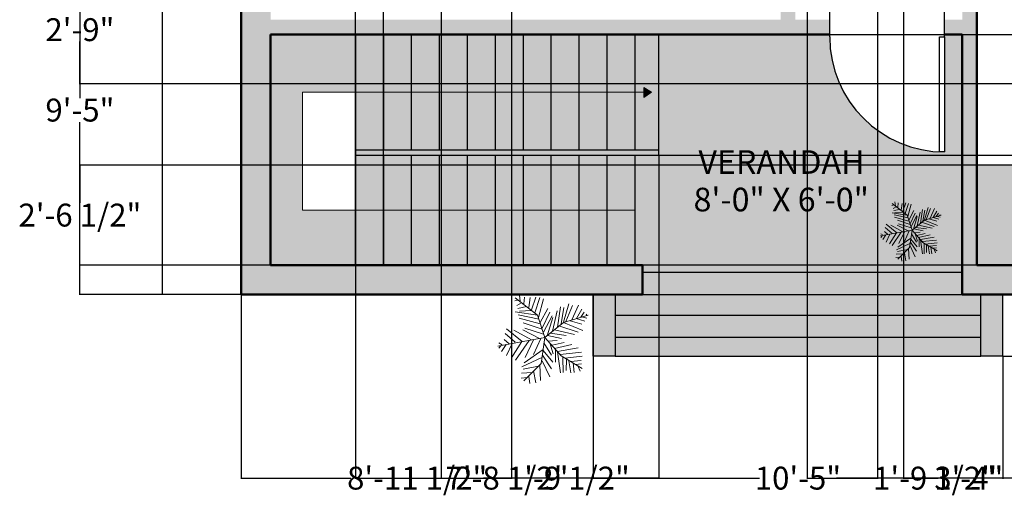
# Model space of a CAD drawing. Units: inches. Extents: x 2974 to 3443, y 2405 to 2963.
# Tile 1 of 13: x 2975 to 3276, y 2405 to 2555. Entities that reach past the tile are written whole.
import ezdxf

# ---------------------------------------------------------------- set-up
doc = ezdxf.new("R2010")
doc.units = ezdxf.units.IN
doc.header["$MEASUREMENT"] = 0
doc.layers.get('0').update_dxf_attribs({"color": 251})
for name, color, linetype, lineweight in [('A-ANNO-DIMS', 2, 'Continuous', 18), ('A-ANNO-SYMB', 250, 'Continuous', 18), ('A-AREA-IDEN', 250, 'Continuous', 25), ('A-DOOR', 32, 'Continuous', 25), ('A-FLOR-CASE', 32, 'Continuous', 25), ('A-FLOR-CASE-PATT', 9, 'Continuous', 13), ('A-FLOR-PATT', 9, 'Continuous', 13), ('A-FLOR-STRS', 250, 'Continuous', 25), ('A-FLOR-STRS-PATT', 254, 'Continuous', 13), ('A-WALL-PATT', 252, 'Continuous', 13), ('greenary', 106, 'Continuous', 13), ('walls', 250, 'Continuous', 50)]:
    doc.layers.add(name, color=color, linetype=linetype, lineweight=lineweight)
doc.styles.get("Standard").update_dxf_attribs({"font": 'arial.ttf'})
doc.dimstyles.get("Standard").update_dxf_attribs({"dimtxt": 7, "dimasz": 0.18, "dimexe": 0.18, "dimexo": 0.0625, "dimgap": 0.09, "dimtad": 0, "dimtih": 1, "dimtoh": 1, "dimzin": 0, "dimdsep": 46, "dimlunit": 3, "dimtxsty": 'Standard', "dimcen": 0.09, "dimadec": 0, "dimazin": 0, "dimtfac": 1, "dimtofl": 0, "dimtmove": 0, "dimatfit": 3, "dimfxl": 1, "dimtolj": 1, "dimtzin": 0, "dimarcsym": 0})

# ---------------------------------------------------------------- blocks, each defined once
blk = doc.blocks.new('*U2')
for p, q in [((0, 0), (0, -6)), ((40, 0), (40, -6))]:
    blk.add_line(p, q)
blk.add_lwpolyline([(0, 0), (0, 40), (1.75, 40), (1.75, 0)], close=True)
blk.add_arc((0, 0), 40, 0, 90)
blk = doc.blocks.new('*U13')
for p, q in [((-8.737, 47.138), (-17.069, 52.711)), ((-10.186, 53.64), (-13.084, 55.962)), ((0, 0), (-10.5, 57)), ((-9.099, 51.782), (-6.563, 55.962)), ((-7.65, 43.423), (-2.578, 49.46)), ((-5.839, 35.992), (4.667, 48.067)), ((-5.114, 28.097), (-24.676, 40.636)), ((-7.288, 39.707), (-21.778, 46.673)), ((-5.114, 27.632), (10.463, 46.673)), ((-2.941, 16.486), (8.652, 37.85)), ((27, 9), (48, 36)), ((27.127, 9.056), (31.112, 35.992)), ((44.153, 36.456), (45.239, 32.741)), ((-31.5, 4.5), (-52.5, 25.5)), ((-48.585, 21.131), (-49.309, 29.026)), ((-43.513, 28.561), (-42.427, 15.558)), ((-38.442, 26.239), (-34.819, 7.663)), ((-35.544, 28.097), (-24.314, 3.947)), ((-14.533, 2.09), (-30.834, 25.31)), ((-3.665, 19.273), (-27.574, 35.527)), ((-24.314, 23.917), (-2.941, 13.7)), ((-1.129, 6.734), (9.014, 26.704)), ((3.942, 1.625), (11.187, 24.381)), ((10.101, 3.483), (17.708, 26.239)), ((16.259, 5.805), (23.142, 31.348)), ((22.055, 7.198), (27.489, 32.277)), ((31.836, 30.883), (32.561, 16.486)), ((35.096, 32.741), (37.27, 22.524)), ((38.719, 34.134), (41.979, 28.561)), ((40.53, 25.775), (48.862, 24.846)), ((43.791, 29.954), (51.036, 30.883)), ((-47.498, 19.737), (-55.83, 18.344)), ((-40.615, 13.7), (-55.105, 10.913)), ((-20.691, 13.7), (-1.129, 4.876)), ((29.662, 12.307), (48.137, 6.269)), ((33.285, 16.486), (48.862, 10.913)), ((36.183, 19.737), (48.137, 17.88)), ((-33.37, 6.269), (-52.207, 5.34)), ((-28.299, 3.483), (-47.86, -5.805)), ((-21.416, 3.018), (-38.079, -8.128)), ((0, 0), (-31.5, 4.5)), ((-15.982, 2.09), (-30.11, -9.521)), ((0, 0), (-22.5, -19.5)), ((-6.563, 1.161), (-21.416, -8.128)), ((0, 0), (27, 9)), ((0, 0), (18, -22.5)), ((6.478, 1.625), (26.04, -8.592)), ((11.187, 3.483), (30.749, -5.805)), ((18.07, 5.805), (35.096, -3.483)), ((24.229, 7.663), (46.688, 1.625)), ((-6.563, -5.805), (-19.967, -9.985)), ((-13.446, -11.378), (-8.737, -32.741)), ((-9.461, -8.592), (-6.201, -23.453)), ((-4.752, -3.483), (-3.665, -14.629)), ((2.493, -3.019), (-1.491, -20.202)), ((1.769, -2.555), (24.229, -9.521)), ((5.029, -6.27), (2.131, -25.775)), ((9.014, -11.378), (3.58, -35.992)), ((7.565, -9.056), (32.198, -14.629)), ((-17.431, -15.094), (-42.789, -18.809)), ((-24.314, -21.596), (-42.427, -22.06)), ((-22.5, -19.5), (-37.5, -45)), ((-15.257, -12.772), (-30.11, -12.772)), ((-20.691, -18.345), (-17.793, -44.352)), ((-17.069, -15.094), (-12.721, -40.172)), ((14.085, -16.951), (6.478, -40.172)), ((18.07, -22.524), (8.289, -45.745)), ((12.274, -15.094), (36.907, -18.809)), ((16.259, -19.738), (36.183, -22.989)), ((18, -22.5), (27, -52.5)), ((18.433, -22.524), (40.53, -29.026)), ((-28.299, -29.026), (-42.789, -31.348)), ((-30.834, -34.135), (-42.427, -35.528)), ((-26.849, -26.24), (-40.253, -25.775)), ((-29.023, -30.884), (-27.936, -43.887)), ((-25.038, -23.918), (-22.865, -45.281)), ((20.244, -30.419), (15.897, -44.816)), ((19.157, -25.311), (38.719, -33.206)), ((21.331, -32.741), (39.081, -40.636)), ((-34.457, -39.708), (-40.978, -42.494)), ((-32.646, -36.921), (-31.921, -44.352)), ((22.78, -37.85), (19.519, -48.532)), ((22.78, -38.314), (34.372, -44.816)), ((24.591, -45.745), (23.142, -50.854)), ((24.591, -43.423), (30.749, -47.603)), ((26.764, -49.925), (28.213, -50.854))]:
    blk.add_line(p, q)
blk = doc.blocks.new('*D20')
at = {"layer": 'A-ANNO-DIMS', "color": 0, "lineweight": -2, "transparency": 16777216}
for p, q in [((3018.41, 2903.19), (3018.14, 2903.19)), ((3018.32, 2903.01), (3018.32, 2690.85)), ((3018.32, 2471.37), (3018.32, 2683.52)), ((3018.41, 2471.19), (3018.14, 2471.19))]:
    blk.add_line(p, q, dxfattribs=at)
at = {"layer": 'A-ANNO-DIMS', "color": 0, "transparency": 16777216}
for points in [[(3018.29, 2903.01), (3018.35, 2903.01), (3018.32, 2903.19)], [(3018.29, 2471.37), (3018.35, 2471.37), (3018.32, 2471.19)]]:
    blk.add_solid(points, dxfattribs=at)
at = {"layer": 'Defpoints', "color": 0, "transparency": 16777216}
for p in [(3018.47, 2903.19), (3018.32, 2471.19), (3018.47, 2471.19)]:
    blk.add_point(p, dxfattribs=at)
at = {"layer": 'A-ANNO-DIMS', "color": 0, "transparency": 16777216, "insert": (3018.32, 2687.19), "char_height": 7, "attachment_point": 5}
blk.add_mtext("\\A1;36'", dxfattribs=at)
blk = doc.blocks.new('*D54')
at = {"layer": 'A-ANNO-DIMS', "color": 0, "lineweight": -2, "transparency": 16777216}
for p, q in [((3042.26, 2583.94), (2992.84, 2583.94)), ((2993.02, 2583.76), (2993.02, 2531.23)), ((2993.02, 2471.37), (2993.02, 2523.9)), ((3042.26, 2471.19), (2992.84, 2471.19))]:
    blk.add_line(p, q, dxfattribs=at)
at = {"layer": 'A-ANNO-DIMS', "color": 0, "transparency": 16777216}
for points in [[(2992.99, 2583.76), (2993.05, 2583.76), (2993.02, 2583.94)], [(2992.99, 2471.37), (2993.05, 2471.37), (2993.02, 2471.19)]]:
    blk.add_solid(points, dxfattribs=at)
at = {"layer": 'Defpoints', "color": 0, "transparency": 16777216}
for p in [(2993.02, 2583.94), (3042.33, 2583.94), (3042.33, 2471.19)]:
    blk.add_point(p, dxfattribs=at)
at = {"layer": 'A-ANNO-DIMS', "color": 0, "transparency": 16777216, "insert": (2993.02, 2527.57), "char_height": 7, "attachment_point": 5}
blk.add_mtext('\\A1;9\'-5"', dxfattribs=at)
blk = doc.blocks.new('*D58')
at = {"layer": 'A-ANNO-DIMS', "color": 0, "lineweight": -2, "transparency": 16777216}
for p, q in [((3042.33, 2471.13), (3042.33, 2414.92)), ((3149.97, 2471.13), (3149.97, 2414.92)), ((3042.51, 2415.1), (3075.87, 2415.1)), ((3149.79, 2415.1), (3116.42, 2415.1))]:
    blk.add_line(p, q, dxfattribs=at)
at = {"layer": 'A-ANNO-DIMS', "color": 0, "transparency": 16777216}
for points in [[(3042.51, 2415.13), (3042.51, 2415.07), (3042.33, 2415.1)], [(3149.79, 2415.13), (3149.79, 2415.07), (3149.97, 2415.1)]]:
    blk.add_solid(points, dxfattribs=at)
at = {"layer": 'Defpoints', "color": 0, "transparency": 16777216}
for p in [(3042.33, 2471.19), (3149.97, 2471.19), (3149.97, 2415.1)]:
    blk.add_point(p, dxfattribs=at)
at = {"layer": 'A-ANNO-DIMS', "color": 0, "transparency": 16777216, "insert": (3096.15, 2415.1), "char_height": 7, "attachment_point": 5}
blk.add_mtext('\\A1;8\'-11 1/2"', dxfattribs=at)
blk = doc.blocks.new('*D59')
at = {"layer": 'A-ANNO-DIMS', "color": 0, "lineweight": -2, "transparency": 16777216}
for p, q in [((3149.97, 2452.35), (3149.97, 2414.92)), ((3275.19, 2452.35), (3275.19, 2414.92)), ((3150.15, 2415.1), (3200.79, 2415.1)), ((3275.01, 2415.1), (3224.36, 2415.1))]:
    blk.add_line(p, q, dxfattribs=at)
at = {"layer": 'A-ANNO-DIMS', "color": 0, "transparency": 16777216}
for points in [[(3150.15, 2415.13), (3150.15, 2415.07), (3149.97, 2415.1)], [(3275.01, 2415.13), (3275.01, 2415.07), (3275.19, 2415.1)]]:
    blk.add_solid(points, dxfattribs=at)
at = {"layer": 'Defpoints', "color": 0, "transparency": 16777216}
for p in [(3149.97, 2452.41), (3275.19, 2452.41), (3275.19, 2415.1)]:
    blk.add_point(p, dxfattribs=at)
at = {"layer": 'A-ANNO-DIMS', "color": 0, "transparency": 16777216, "insert": (3212.58, 2415.1), "char_height": 7, "attachment_point": 5}
blk.add_mtext('\\A1;10\'-5"', dxfattribs=at)
blk = doc.blocks.new('*D60')
at = {"layer": 'A-ANNO-DIMS', "color": 0, "lineweight": -2, "transparency": 16777216}
for p, q in [((3275.25, 2471.19), (3409.82, 2471.19)), ((3409.64, 2471.01), (3409.64, 2465.41)), ((3409.64, 2452.59), (3409.64, 2458.2)), ((3275.25, 2452.41), (3409.82, 2452.41))]:
    blk.add_line(p, q, dxfattribs=at)
at = {"layer": 'A-ANNO-DIMS', "color": 0, "transparency": 16777216}
for points in [[(3409.61, 2471.01), (3409.67, 2471.01), (3409.64, 2471.19)], [(3409.61, 2452.59), (3409.67, 2452.59), (3409.64, 2452.41)]]:
    blk.add_solid(points, dxfattribs=at)
at = {"layer": 'Defpoints', "color": 0, "transparency": 16777216}
for p in [(3275.19, 2471.19), (3409.64, 2471.19), (3275.19, 2452.41)]:
    blk.add_point(p, dxfattribs=at)
at = {"layer": 'A-ANNO-DIMS', "color": 0, "transparency": 16777216, "insert": (3409.64, 2461.8), "char_height": 7, "attachment_point": 5}
blk.add_mtext('\\A1;1\'-7"', dxfattribs=at)
blk = doc.blocks.new('*D61')
at = {"layer": 'A-ANNO-DIMS', "color": 0, "lineweight": -2, "transparency": 16777216}
for p, q in [((3222.29, 2555.25), (3222.29, 2952.68)), ((3222.47, 2952.5), (3227.69, 2952.5)), ((3257.25, 2952.5), (3252.03, 2952.5)), ((3257.43, 2555.25), (3257.43, 2952.68))]:
    blk.add_line(p, q, dxfattribs=at)
at = {"layer": 'A-ANNO-DIMS', "color": 0, "transparency": 16777216}
for points in [[(3222.47, 2952.53), (3222.47, 2952.47), (3222.29, 2952.5)], [(3257.25, 2952.53), (3257.25, 2952.47), (3257.43, 2952.5)]]:
    blk.add_solid(points, dxfattribs=at)
at = {"layer": 'Defpoints', "color": 0, "transparency": 16777216}
for p in [(3257.43, 2952.5), (3222.29, 2555.19), (3257.43, 2555.19)]:
    blk.add_point(p, dxfattribs=at)
at = {"layer": 'A-ANNO-DIMS', "color": 0, "transparency": 16777216, "insert": (3239.86, 2952.5), "char_height": 7, "attachment_point": 5}
blk.add_mtext('\\A1;2\'-11"', dxfattribs=at)
blk = doc.blocks.new('*D63')
at = {"layer": 'A-ANNO-DIMS', "color": 0, "lineweight": -2, "transparency": 16777216}
for p, q in [((3244.83, 2751.13), (3244.83, 2414.92)), ((3284.83, 2751.13), (3284.83, 2414.92)), ((3245.01, 2415.1), (3255.43, 2415.1)), ((3284.65, 2415.1), (3274.22, 2415.1))]:
    blk.add_line(p, q, dxfattribs=at)
at = {"layer": 'A-ANNO-DIMS', "color": 0, "transparency": 16777216}
for points in [[(3245.01, 2415.13), (3245.01, 2415.07), (3244.83, 2415.1)], [(3284.65, 2415.13), (3284.65, 2415.07), (3284.83, 2415.1)]]:
    blk.add_solid(points, dxfattribs=at)
at = {"layer": 'Defpoints', "color": 0, "transparency": 16777216}
for p in [(3244.83, 2751.19), (3284.83, 2751.19), (3284.83, 2415.1)]:
    blk.add_point(p, dxfattribs=at)
at = {"layer": 'A-ANNO-DIMS', "color": 0, "transparency": 16777216, "insert": (3264.83, 2415.1), "char_height": 7, "attachment_point": 5}
blk.add_mtext('\\A1;3\'-4"', dxfattribs=at)
blk = doc.blocks.new('*D64')
at = {"layer": 'A-ANNO-DIMS', "color": 0, "lineweight": -2, "transparency": 16777216}
for p, q in [((3103.48, 2840.13), (3103.48, 2414.92)), ((3124.99, 2840.13), (3124.99, 2414.92)), ((3103.66, 2415.1), (3124.81, 2415.1)), ((3124.99, 2415.1), (3125.17, 2415.1))]:
    blk.add_line(p, q, dxfattribs=at)
at = {"layer": 'A-ANNO-DIMS', "color": 0, "transparency": 16777216}
for points in [[(3103.66, 2415.13), (3103.66, 2415.07), (3103.48, 2415.1)], [(3124.81, 2415.13), (3124.81, 2415.07), (3124.99, 2415.1)]]:
    blk.add_solid(points, dxfattribs=at)
at = {"layer": 'Defpoints', "color": 0, "transparency": 16777216}
for p in [(3103.48, 2840.19), (3124.99, 2840.19), (3124.99, 2415.1)]:
    blk.add_point(p, dxfattribs=at)
at = {"layer": 'A-ANNO-DIMS', "color": 0, "transparency": 16777216, "insert": (3142.39, 2415.1), "char_height": 7, "attachment_point": 5}
blk.add_mtext('\\A1;1\'-9 1/2"', dxfattribs=at)
blk = doc.blocks.new('*D65')
at = {"layer": 'A-ANNO-DIMS', "color": 0, "lineweight": -2, "transparency": 16777216}
for p, q in [((3215.45, 2808.13), (3215.45, 2414.92)), ((3236.95, 2808.13), (3236.95, 2414.92)), ((3215.63, 2415.1), (3236.77, 2415.1)), ((3236.95, 2415.1), (3237.13, 2415.1))]:
    blk.add_line(p, q, dxfattribs=at)
at = {"layer": 'A-ANNO-DIMS', "color": 0, "transparency": 16777216}
for points in [[(3215.63, 2415.13), (3215.63, 2415.07), (3215.45, 2415.1)], [(3236.77, 2415.13), (3236.77, 2415.07), (3236.95, 2415.1)]]:
    blk.add_solid(points, dxfattribs=at)
at = {"layer": 'Defpoints', "color": 0, "transparency": 16777216}
for p in [(3215.45, 2808.19), (3236.95, 2808.19), (3236.95, 2415.1)]:
    blk.add_point(p, dxfattribs=at)
at = {"layer": 'A-ANNO-DIMS', "color": 0, "transparency": 16777216, "insert": (3254.35, 2415.1), "char_height": 7, "attachment_point": 5}
blk.add_mtext('\\A1;1\'-9 1/2"', dxfattribs=at)
blk = doc.blocks.new('*D66')
at = {"layer": 'A-ANNO-DIMS', "color": 0, "lineweight": -2, "transparency": 16777216}
for p, q in [((3077.27, 2513.73), (3077.27, 2414.92)), ((3170, 2513.73), (3170, 2414.92)), ((3077.45, 2415.1), (3106.11, 2415.1)), ((3169.82, 2415.1), (3141.16, 2415.1))]:
    blk.add_line(p, q, dxfattribs=at)
at = {"layer": 'A-ANNO-DIMS', "color": 0, "transparency": 16777216}
for points in [[(3077.45, 2415.13), (3077.45, 2415.07), (3077.27, 2415.1)], [(3169.82, 2415.13), (3169.82, 2415.07), (3170, 2415.1)]]:
    blk.add_solid(points, dxfattribs=at)
at = {"layer": 'Defpoints', "color": 0, "transparency": 16777216}
for p in [(3077.27, 2513.79), (3170, 2513.79), (3170, 2415.1)]:
    blk.add_point(p, dxfattribs=at)
at = {"layer": 'A-ANNO-DIMS', "color": 0, "transparency": 16777216, "insert": (3123.64, 2415.1), "char_height": 7, "attachment_point": 5}
blk.add_mtext('\\A1;7\'-8 1/2"', dxfattribs=at)
blk = doc.blocks.new('*D67')
at = {"layer": 'A-ANNO-DIMS', "color": 0, "lineweight": -2, "transparency": 16777216}
for p, q in [((3170.07, 2550.69), (3409.82, 2550.69)), ((3409.64, 2550.51), (3409.64, 2535.9)), ((3409.64, 2513.97), (3409.64, 2528.57)), ((3170.07, 2513.79), (3409.82, 2513.79))]:
    blk.add_line(p, q, dxfattribs=at)
at = {"layer": 'A-ANNO-DIMS', "color": 0, "transparency": 16777216}
for points in [[(3409.61, 2550.51), (3409.67, 2550.51), (3409.64, 2550.69)], [(3409.61, 2513.97), (3409.67, 2513.97), (3409.64, 2513.79)]]:
    blk.add_solid(points, dxfattribs=at)
at = {"layer": 'Defpoints', "color": 0, "transparency": 16777216}
for p in [(3170, 2550.69), (3409.64, 2550.69), (3170, 2513.79)]:
    blk.add_point(p, dxfattribs=at)
at = {"layer": 'A-ANNO-DIMS', "color": 0, "transparency": 16777216, "insert": (3409.64, 2532.24), "char_height": 7, "attachment_point": 5}
blk.add_mtext('\\A1;3\'-1"', dxfattribs=at)
blk = doc.blocks.new('*D68')
at = {"layer": 'A-ANNO-DIMS', "color": 0, "lineweight": -2, "transparency": 16777216}
for p, q in [((3077.27, 2480.25), (3077.27, 2952.68)), ((3077.45, 2952.5), (3085.63, 2952.5)), ((3085.81, 2480.25), (3085.81, 2952.68)), ((3085.81, 2952.5), (3085.99, 2952.5))]:
    blk.add_line(p, q, dxfattribs=at)
at = {"layer": 'A-ANNO-DIMS', "color": 0, "transparency": 16777216}
for points in [[(3077.45, 2952.53), (3077.45, 2952.47), (3077.27, 2952.5)], [(3085.63, 2952.53), (3085.63, 2952.47), (3085.81, 2952.5)]]:
    blk.add_solid(points, dxfattribs=at)
at = {"layer": 'Defpoints', "color": 0, "transparency": 16777216}
for p in [(3085.81, 2952.5), (3077.27, 2480.19), (3085.81, 2480.19)]:
    blk.add_point(p, dxfattribs=at)
at = {"layer": 'A-ANNO-DIMS', "color": 0, "transparency": 16777216, "insert": (3103.54, 2952.5), "char_height": 7, "attachment_point": 5}
blk.add_mtext('\\A1;0\'-8 1/2"', dxfattribs=at)
blk = doc.blocks.new('*D71')
at = {"layer": 'A-ANNO-DIMS', "color": 0, "lineweight": -2, "transparency": 16777216}
for p, q in [((3267.26, 2510.76), (2992.84, 2510.76)), ((2993.02, 2510.58), (2993.02, 2499.18)), ((2993.02, 2480.37), (2993.02, 2491.77)), ((3267.26, 2480.19), (2992.84, 2480.19))]:
    blk.add_line(p, q, dxfattribs=at)
at = {"layer": 'A-ANNO-DIMS', "color": 0, "transparency": 16777216}
for points in [[(2992.99, 2510.58), (2993.05, 2510.58), (2993.02, 2510.76)], [(2992.99, 2480.37), (2993.05, 2480.37), (2993.02, 2480.19)]]:
    blk.add_solid(points, dxfattribs=at)
at = {"layer": 'Defpoints', "color": 0, "transparency": 16777216}
for p in [(2993.02, 2510.76), (3267.33, 2510.76), (3267.33, 2480.19)]:
    blk.add_point(p, dxfattribs=at)
at = {"layer": 'A-ANNO-DIMS', "color": 0, "transparency": 16777216, "insert": (2993.02, 2495.48), "char_height": 7, "attachment_point": 5}
blk.add_mtext('\\A1;2\'-6 1/2"', dxfattribs=at)
blk = doc.blocks.new('*D76')
at = {"layer": 'A-ANNO-DIMS', "color": 0, "lineweight": -2, "transparency": 16777216}
for p, q in [((3352.84, 2568.64), (2992.84, 2568.64)), ((2993.02, 2568.46), (2993.02, 2555.8)), ((2993.02, 2535.82), (2993.02, 2548.48)), ((3352.84, 2535.64), (2992.84, 2535.64))]:
    blk.add_line(p, q, dxfattribs=at)
at = {"layer": 'A-ANNO-DIMS', "color": 0, "transparency": 16777216}
for points in [[(2992.99, 2568.46), (2993.05, 2568.46), (2993.02, 2568.64)], [(2992.99, 2535.82), (2993.05, 2535.82), (2993.02, 2535.64)]]:
    blk.add_solid(points, dxfattribs=at)
at = {"layer": 'Defpoints', "color": 0, "transparency": 16777216}
for p in [(2993.02, 2568.64), (3352.9, 2568.64), (3352.9, 2535.64)]:
    blk.add_point(p, dxfattribs=at)
at = {"layer": 'A-ANNO-DIMS', "color": 0, "transparency": 16777216, "insert": (2993.02, 2552.14), "char_height": 7, "attachment_point": 5}
blk.add_mtext('\\A1;2\'-9"', dxfattribs=at)
blk = doc.blocks.new('*D78')
at = {"layer": 'A-ANNO-DIMS', "color": 0, "lineweight": -2, "transparency": 16777216}
for p, q in [((3267.33, 2480.25), (3267.33, 2952.68)), ((3267.51, 2952.5), (3271.55, 2952.5)), ((3310.68, 2952.5), (3306.64, 2952.5)), ((3310.86, 2481.93), (3310.86, 2952.68))]:
    blk.add_line(p, q, dxfattribs=at)
at = {"layer": 'A-ANNO-DIMS', "color": 0, "transparency": 16777216}
for points in [[(3267.51, 2952.53), (3267.51, 2952.47), (3267.33, 2952.5)], [(3310.68, 2952.53), (3310.68, 2952.47), (3310.86, 2952.5)]]:
    blk.add_solid(points, dxfattribs=at)
at = {"layer": 'Defpoints', "color": 0, "transparency": 16777216}
for p in [(3310.86, 2952.5), (3310.86, 2481.87), (3267.33, 2480.19)]:
    blk.add_point(p, dxfattribs=at)
at = {"layer": 'A-ANNO-DIMS', "color": 0, "transparency": 16777216, "insert": (3289.09, 2952.5), "char_height": 7, "attachment_point": 5}
blk.add_mtext('\\A1;3\'-7 1/2"', dxfattribs=at)

msp = doc.modelspace()

# ---------------------------------------------------------------- hatches: boundary and pattern name
at = {"layer": 'A-ANNO-SYMB'}
h = msp.add_hatch(color=256, dxfattribs=at)
h.dxf.hatch_style = 1
h.paths.add_polyline_path([(3165.474, 2534.508), (3165.474, 2533.04), (3165.474, 2531.431), (3167.838, 2533.04)])
at = {"layer": 'A-FLOR-CASE-PATT'}
h = msp.add_hatch(color=256, dxfattribs=at)
h.dxf.hatch_style = 1
h.paths.add_polyline_path([(3375.326, 2480.188), (3267.326, 2480.188), (3267.326, 2510.762), (3342.691, 2510.762), (3342.691, 2604.688), (3375.326, 2604.688)])
h.paths.add_polyline_path([(3332.464, 2481.869, -0.4142136), (3331.564, 2480.969), (3311.764, 2480.969, -0.4142136), (3310.864, 2481.869), (3310.864, 2501.669, -0.4142136), (3311.764, 2502.569), (3331.564, 2502.569, -0.4142136), (3332.464, 2501.669)], flags=16)
h.paths.add_polyline_path([(3324.078, 2497.114), (3323.628, 2497.114, -0.0171907), (3323.627, 2497.339), (3324.077, 2497.339, -0.9825922), (3329.722, 2497.24, -0.9779445)], flags=0)
h.paths.add_polyline_path([(3328.474, 2497.24, -1), (3325.324, 2497.24, -1)], flags=0)
h.paths.add_polyline_path([(3326.899, 2496.115, -1), (3326.899, 2498.365, -1)], flags=0)
h.paths.add_polyline_path([(3326.899, 2496.453, -1), (3326.899, 2498.028, -1)], flags=0)
h.paths.add_polyline_path([(3329.722, 2486.666, -0.9779445), (3324.078, 2486.54), (3323.628, 2486.54, -0.0171907), (3323.627, 2486.765), (3324.077, 2486.765, -0.9825922)], flags=0)
h.paths.add_polyline_path([(3328.474, 2486.666, -1), (3325.324, 2486.666, -1)], flags=0)
h.paths.add_polyline_path([(3326.899, 2485.541, -1), (3326.899, 2487.791, -1)], flags=0)
h.paths.add_polyline_path([(3326.899, 2485.878, -1), (3326.899, 2487.453, -1)], flags=0)
h.paths.add_polyline_path([(3323.167, 2491.769, -1), (3320.16, 2491.769, -1)], flags=0)
h.paths.add_polyline_path([(3318.032, 2494.858), (3318.257, 2494.468, -0.0171907), (3318.063, 2494.355), (3317.838, 2494.745, -0.5505708), (3313.696, 2497.114), (3313.246, 2497.114, -0.0171907), (3313.245, 2497.339), (3313.695, 2497.339, -0.6105283), (3318.24, 2499.476), (3318.53, 2499.821, -0.0171906), (3318.702, 2499.677), (3318.413, 2499.332, -0.2116406), (3319.34, 2497.24, -0.2564461)], flags=0)
h.paths.add_polyline_path([(3314.942, 2497.24, -1), (3318.092, 2497.24, -1)], flags=0)
h.paths.add_polyline_path([(3316.517, 2496.115, -1), (3316.517, 2498.365, -1)], flags=0)
h.paths.add_polyline_path([(3318.817, 2489.141), (3318.528, 2488.796, -0.2116406), (3319.454, 2486.704, -0.2564461), (3318.147, 2484.322), (3318.372, 2483.932, -0.0171907), (3318.177, 2483.819), (3317.952, 2484.209, -0.5505708), (3313.811, 2486.578), (3313.361, 2486.578, -0.0171907), (3313.36, 2486.803), (3313.81, 2486.803, -0.6105283), (3318.355, 2488.94), (3318.645, 2489.285, -0.0171906)], flags=0)
h.paths.add_polyline_path([(3316.517, 2496.453, -1), (3316.517, 2498.028, -1)], flags=0)
h.paths.add_polyline_path([(3318.206, 2486.704, -1), (3315.056, 2486.704, -1)], flags=0)
h.paths.add_polyline_path([(3316.631, 2485.579, -1), (3316.631, 2487.829, -1)], flags=0)
h.paths.add_polyline_path([(3316.631, 2485.917, -1), (3316.631, 2487.492, -1)], flags=0)
h.paths.add_polyline_path([(3351.404, 2537.14), (3351.404, 2567.14, -0.4142136), (3352.904, 2568.64), (3371.904, 2568.64, -0.4142136), (3373.404, 2567.14), (3373.404, 2537.14, -0.4142136), (3371.904, 2535.64), (3352.904, 2535.64, -0.4142136)], flags=16)
h.paths.add_polyline_path([(3352.904, 2540.14), (3352.904, 2548.14, -0.4142136), (3355.904, 2551.14), (3366.404, 2551.14, -0.4142136), (3369.404, 2548.14), (3369.404, 2540.14, -0.4142136), (3366.404, 2537.14), (3355.904, 2537.14, -0.4142136)], flags=0)
h.paths.add_polyline_path([(3362.154, 2544.39, -1), (3364.654, 2544.39, -1)], flags=0)
h.paths.add_polyline_path([(3369.904, 2549.14, -1), (3371.904, 2549.14, -1)], flags=0)
h.paths.add_polyline_path([(3370.523, 2553.675, -0.4631995), (3371.039, 2552.239), (3370.636, 2551.542, -0.4369422), (3369.205, 2551.215), (3363.226, 2555.707), (3363.726, 2556.573)], flags=0)
h.paths.add_polyline_path([(3369.904, 2555.14, -1), (3371.904, 2555.14, -1)], flags=0)
h.paths.add_polyline_path([(3362.154, 2559.89, -1), (3364.654, 2559.89, -1)], flags=0)
at = {"layer": 'A-FLOR-PATT'}
h = msp.add_hatch(color=256, dxfattribs=at)
h.dxf.hatch_style = 1
h.paths.add_polyline_path([(3222.294, 2549.918), (3222.294, 2550.688), (3170.003, 2550.688), (3170.003, 2515.438), (3170.003, 2513.788), (3162.699, 2513.788), (3162.699, 2480.188), (3165.027, 2480.188), (3165.027, 2478.063), (3262.826, 2478.063), (3262.826, 2550.688), (3257.429, 2550.688), (3257.429, 2549.918), (3257.429, 2514.783), (3255.892, 2514.783), (3255.892, 2514.817, -0.4014527)])
h.paths.add_polyline_path([(3253.947, 2494.738), (3253.965, 2494.732), (3253.972, 2494.746)], flags=16)
h.paths.add_polyline_path([(3245.908, 2495.495), (3245.933, 2495.491), (3247.469, 2490.884), (3247.922, 2491.246), (3247.944, 2491.316), (3247.994, 2491.304), (3251.267, 2493.923), (3251.278, 2493.96), (3251.302, 2493.95), (3247.469, 2490.884), (3249.988, 2487.977), (3250.024, 2487.983), (3250.032, 2487.926), (3247.469, 2490.884), (3242.689, 2490.003), (3242.723, 2490.058), (3242.771, 2490.018), (3247.469, 2490.884), (3245.94, 2495.47), (3244.722, 2496.417), (3244.624, 2496.412), (3244.646, 2496.476)], flags=16)
h.paths.add_polyline_path([(3178.822, 2494.649), (3235.064, 2494.649), (3235.064, 2505.719), (3178.822, 2505.719)], flags=24)
h.paths.add_polyline_path([(3180.338, 2506.28), (3240.053, 2506.28), (3240.053, 2517.121), (3180.338, 2517.121)], flags=24)
at = {"layer": 'A-FLOR-STRS-PATT'}
h = msp.add_hatch(color=256, dxfattribs=at)
h.dxf.hatch_style = 1
h.paths.add_polyline_path([(3077.267, 2550.688), (3051.326, 2550.688), (3051.326, 2480.188), (3077.267, 2480.188), (3077.267, 2496.988), (3061.108, 2496.988), (3061.108, 2533.04), (3077.267, 2533.04)])
h.paths.add_polyline_path([(3085.81, 2550.688), (3077.267, 2550.688), (3077.267, 2533.04), (3085.81, 2533.04)])
h.paths.add_polyline_path([(3094.353, 2550.688), (3085.81, 2550.688), (3085.81, 2533.04), (3094.353, 2533.04)])
h.paths.add_polyline_path([(3102.896, 2550.688), (3094.353, 2550.688), (3094.353, 2533.04), (3102.896, 2533.04)])
h.paths.add_polyline_path([(3085.81, 2533.04), (3077.267, 2533.04), (3077.267, 2515.438), (3085.81, 2515.438)])
h.paths.add_polyline_path([(3094.353, 2533.04), (3085.81, 2533.04), (3085.81, 2515.438), (3094.353, 2515.438)])
h.paths.add_polyline_path([(3102.896, 2533.04), (3094.353, 2533.04), (3094.353, 2515.438), (3102.896, 2515.438)])
h.paths.add_polyline_path([(3111.44, 2533.04), (3102.896, 2533.04), (3102.896, 2515.438), (3111.44, 2515.438)])
h.paths.add_polyline_path([(3119.983, 2533.04), (3111.44, 2533.04), (3111.44, 2515.438), (3119.983, 2515.438)])
h.paths.add_polyline_path([(3128.526, 2533.04), (3119.983, 2533.04), (3119.983, 2515.438), (3128.526, 2515.438)])
h.paths.add_polyline_path([(3137.069, 2533.04), (3128.526, 2533.04), (3128.526, 2515.438), (3137.069, 2515.438)])
h.paths.add_polyline_path([(3145.612, 2533.04), (3137.069, 2533.04), (3137.069, 2515.438), (3145.612, 2515.438)])
h.paths.add_polyline_path([(3154.155, 2533.04), (3145.612, 2533.04), (3145.612, 2515.438), (3154.155, 2515.438)])
h.paths.add_polyline_path([(3162.699, 2533.04), (3154.155, 2533.04), (3154.155, 2515.438), (3162.699, 2515.438)])
h.paths.add_polyline_path([(3170.003, 2550.688), (3162.699, 2550.688), (3162.699, 2533.04), (3165.474, 2533.04), (3165.474, 2534.508), (3167.838, 2533.04), (3165.474, 2531.431), (3165.474, 2533.04), (3162.699, 2533.04), (3162.699, 2515.438), (3170.003, 2515.438)])
h.paths.add_polyline_path([(3162.699, 2550.688), (3154.155, 2550.688), (3154.155, 2533.04), (3162.699, 2533.04)])
h.paths.add_polyline_path([(3154.155, 2550.688), (3145.612, 2550.688), (3145.612, 2533.04), (3154.155, 2533.04)])
h.paths.add_polyline_path([(3145.612, 2550.688), (3137.069, 2550.688), (3137.069, 2533.04), (3145.612, 2533.04)])
h.paths.add_polyline_path([(3137.069, 2550.688), (3128.526, 2550.688), (3128.526, 2533.04), (3137.069, 2533.04)])
h.paths.add_polyline_path([(3128.526, 2550.688), (3119.983, 2550.688), (3119.983, 2533.04), (3128.526, 2533.04)])
h.paths.add_polyline_path([(3111.44, 2550.688), (3102.896, 2550.688), (3102.896, 2533.04), (3111.44, 2533.04)])
h.paths.add_polyline_path([(3119.983, 2550.688), (3111.44, 2550.688), (3111.44, 2533.04), (3119.983, 2533.04)])
h = msp.add_hatch(color=256, dxfattribs=at)
h.dxf.hatch_style = 1
h.paths.add_polyline_path([(3170.003, 2515.438), (3077.267, 2515.438), (3077.267, 2513.788), (3170.003, 2513.788)])
h = msp.add_hatch(color=256, dxfattribs=at)
h.dxf.hatch_style = 1
h.paths.add_polyline_path([(3085.81, 2513.788), (3077.267, 2513.788), (3077.267, 2496.988), (3085.81, 2496.988)])
h.paths.add_polyline_path([(3085.81, 2496.988), (3077.267, 2496.988), (3077.267, 2480.188), (3085.81, 2480.188)])
h.paths.add_polyline_path([(3094.353, 2513.788), (3085.81, 2513.788), (3085.81, 2496.988), (3094.353, 2496.988)])
h.paths.add_polyline_path([(3094.353, 2496.988), (3085.81, 2496.988), (3085.81, 2480.188), (3094.353, 2480.188)])
h.paths.add_polyline_path([(3111.44, 2513.788), (3102.896, 2513.788), (3102.896, 2496.988), (3111.44, 2496.988)])
h.paths.add_polyline_path([(3102.896, 2496.988), (3094.353, 2496.988), (3094.353, 2480.188), (3102.896, 2480.188)])
h.paths.add_polyline_path([(3102.896, 2513.788), (3094.353, 2513.788), (3094.353, 2496.988), (3102.896, 2496.988)])
h.paths.add_polyline_path([(3111.44, 2496.988), (3102.896, 2496.988), (3102.896, 2480.188), (3111.44, 2480.188)])
h.paths.add_polyline_path([(3119.983, 2513.788), (3111.44, 2513.788), (3111.44, 2496.988), (3119.983, 2496.988)])
h.paths.add_polyline_path([(3119.983, 2496.988), (3111.44, 2496.988), (3111.44, 2480.188), (3119.983, 2480.188)])
h.paths.add_polyline_path([(3128.526, 2513.788), (3119.983, 2513.788), (3119.983, 2496.988), (3128.526, 2496.988)])
h.paths.add_polyline_path([(3128.526, 2496.988), (3119.983, 2496.988), (3119.983, 2480.188), (3128.526, 2480.188)])
h.paths.add_polyline_path([(3137.069, 2513.788), (3128.526, 2513.788), (3128.526, 2496.988), (3137.069, 2496.988)])
h.paths.add_polyline_path([(3145.612, 2496.988), (3137.069, 2496.988), (3137.069, 2480.188), (3145.612, 2480.188)])
h.paths.add_polyline_path([(3145.612, 2513.788), (3137.069, 2513.788), (3137.069, 2496.988), (3145.612, 2496.988)])
h.paths.add_polyline_path([(3137.069, 2496.988), (3128.526, 2496.988), (3128.526, 2480.188), (3137.069, 2480.188)])
h.paths.add_polyline_path([(3154.155, 2513.788), (3145.612, 2513.788), (3145.612, 2496.988), (3154.155, 2496.988)])
h.paths.add_polyline_path([(3154.155, 2496.988), (3145.612, 2496.988), (3145.612, 2480.188), (3154.155, 2480.188)])
h.paths.add_polyline_path([(3162.699, 2513.788), (3154.155, 2513.788), (3154.155, 2496.988), (3162.699, 2496.988)])
h.paths.add_polyline_path([(3162.699, 2496.988), (3154.155, 2496.988), (3154.155, 2480.188), (3162.699, 2480.188)])
h = msp.add_hatch(color=256, dxfattribs=at)
h.dxf.hatch_style = 1
h.paths.add_polyline_path([(3262.826, 2478.063), (3165.027, 2478.063), (3165.027, 2471.188), (3262.826, 2471.188)])
h.paths.add_polyline_path([(3268.471, 2471.188), (3262.826, 2471.188), (3165.027, 2471.188), (3156.684, 2471.188), (3156.684, 2464.944), (3268.471, 2464.944)])
h.paths.add_polyline_path([(3268.471, 2464.944), (3156.684, 2464.944), (3156.684, 2458.196), (3268.471, 2458.196)])
h.paths.add_polyline_path([(3268.471, 2455.229), (3268.471, 2458.196), (3156.684, 2458.196), (3156.684, 2452.413), (3268.471, 2452.413)])
at = {"layer": 'A-WALL-PATT'}
h = msp.add_hatch(color=256, dxfattribs=at)
h.dxf.hatch_style = 1
h.paths.add_polyline_path([(3222.294, 2555.188), (3211.826, 2555.188), (3211.826, 2657.938), (3207.326, 2657.938), (3207.326, 2555.188), (3051.326, 2555.188), (3051.326, 2583.943), (3042.326, 2583.943), (3042.326, 2471.188), (3165.027, 2471.188), (3165.027, 2480.188), (3051.326, 2480.188), (3051.326, 2550.688), (3222.294, 2550.688)])
h.paths.add_polyline_path([(3188.326, 2700.207), (3183.826, 2700.207), (3183.826, 2691.688), (3051.326, 2691.688), (3051.326, 2740.572), (3042.326, 2740.572), (3042.326, 2651.235), (3045.517, 2651.235), (3051.326, 2651.235), (3051.326, 2687.188), (3188.326, 2687.188)])
h.paths.add_polyline_path([(3051.326, 2894.188), (3074.298, 2894.188), (3074.298, 2903.188), (3042.326, 2903.188), (3042.326, 2807.864), (3045.517, 2807.864), (3051.326, 2807.864), (3051.326, 2835.688), (3103.457, 2835.688), (3103.457, 2839.066, -0.0124729), (3103.485, 2840.188), (3051.326, 2840.188)])
h.paths.add_polyline_path([(3201.987, 2903.188), (3100.263, 2903.188), (3100.263, 2894.188), (3131.326, 2894.188), (3131.326, 2835.688), (3135.826, 2835.688), (3135.826, 2894.188), (3183.826, 2894.188), (3183.826, 2840.188), (3159.826, 2840.188), (3159.826, 2835.688), (3183.826, 2835.688), (3183.826, 2740.207), (3188.326, 2740.207), (3188.326, 2803.688), (3215.422, 2803.688), (3215.422, 2807.066, -0.0124729), (3215.45, 2808.188), (3188.326, 2808.188), (3188.326, 2894.188), (3201.987, 2894.188)])
h.paths.add_polyline_path([(3283.564, 2903.188), (3227.952, 2903.188), (3227.952, 2894.188), (3240.326, 2894.188), (3240.326, 2755.688), (3188.326, 2755.688), (3188.326, 2751.188), (3244.826, 2751.188), (3244.826, 2757.188), (3244.826, 2797.188), (3244.826, 2894.188), (3283.564, 2894.188)])
h.paths.add_polyline_path([(3384.326, 2903.188), (3346.694, 2903.188), (3346.694, 2894.188), (3375.326, 2894.188), (3375.326, 2755.688), (3284.826, 2755.688), (3284.826, 2751.188), (3375.326, 2751.188), (3375.326, 2710.653), (3378.517, 2710.653), (3384.326, 2710.653)])
h.paths.add_polyline_path([(3384.326, 2643.361), (3375.326, 2643.361), (3375.326, 2609.188), (3330.003, 2609.188), (3330.003, 2604.688), (3375.326, 2604.688), (3375.326, 2480.188), (3356.49, 2480.188), (3356.49, 2471.188), (3384.326, 2471.188)])
h.paths.add_polyline_path([(3267.326, 2609.188), (3262.826, 2609.188), (3262.826, 2555.188), (3257.429, 2555.188), (3257.429, 2550.688), (3262.826, 2550.688), (3262.826, 2471.188), (3293.36, 2471.188), (3293.36, 2480.188), (3267.326, 2480.188)])
h.paths.add_polyline_path([(3275.186, 2471.188), (3268.471, 2471.188), (3268.471, 2455.229), (3268.471, 2452.413), (3275.186, 2452.413)])
h.paths.add_polyline_path([(3156.684, 2471.188), (3149.969, 2471.188), (3149.969, 2452.413), (3156.684, 2452.413)])

# ---------------------------------------------------------------- linework, layer by layer
at = {"layer": 'A-ANNO-SYMB'}
for p, q in [((3061.108, 2496.988), (3061.108, 2533.04)), ((3061.108, 2533.04), (3165.474, 2533.04)), ((3165.474, 2533.04), (3165.474, 2534.508)), ((3165.474, 2534.508), (3167.838, 2533.04)), ((3167.838, 2533.04), (3165.474, 2531.431)), ((3165.474, 2531.431), (3165.474, 2533.04)), ((3162.699, 2496.988), (3061.108, 2496.988))]:
    msp.add_line(p, q, dxfattribs=at)
at = {"layer": 'A-FLOR-CASE'}
msp.add_line((3342.691, 2510.762), (3267.326, 2510.762), dxfattribs=at)
at = {"layer": 'A-FLOR-STRS'}
for p, q in [((3077.267, 2550.688), (3077.267, 2480.188)), ((3085.81, 2550.688), (3085.81, 2515.438)), ((3094.353, 2550.688), (3094.353, 2515.438)), ((3102.896, 2550.688), (3102.896, 2515.438)), ((3111.44, 2550.688), (3111.44, 2515.438)), ((3119.983, 2550.688), (3119.983, 2515.438)), ((3128.526, 2550.688), (3128.526, 2515.438)), ((3137.069, 2550.688), (3137.069, 2515.438)), ((3145.612, 2550.688), (3145.612, 2515.438)), ((3154.155, 2550.688), (3154.155, 2515.438)), ((3162.699, 2550.688), (3162.699, 2515.438)), ((3170.003, 2515.438), (3170.003, 2550.688)), ((3077.267, 2515.438), (3170.003, 2515.438)), ((3170.003, 2513.788), (3170.003, 2515.438)), ((3077.267, 2513.788), (3170.003, 2513.788)), ((3085.81, 2513.788), (3085.81, 2480.188)), ((3094.353, 2513.788), (3094.353, 2480.188)), ((3102.896, 2513.788), (3102.896, 2480.188)), ((3111.44, 2513.788), (3111.44, 2480.188)), ((3119.983, 2513.788), (3119.983, 2480.188)), ((3128.526, 2513.788), (3128.526, 2480.188)), ((3137.069, 2513.788), (3137.069, 2480.188)), ((3145.612, 2513.788), (3145.612, 2480.188)), ((3154.155, 2513.788), (3154.155, 2480.188)), ((3162.699, 2513.788), (3162.699, 2480.188)), ((3165.027, 2478.063), (3262.826, 2478.063)), ((3149.969, 2452.413), (3149.969, 2471.188)), ((3156.684, 2471.188), (3156.684, 2452.413)), ((3165.027, 2471.188), (3262.826, 2471.188)), ((3268.471, 2455.229), (3268.471, 2471.188)), ((3275.186, 2471.188), (3275.186, 2452.413)), ((3156.684, 2464.944), (3268.471, 2464.944)), ((3156.684, 2458.196), (3268.471, 2458.196)), ((3268.471, 2452.413), (3268.471, 2455.229)), ((3156.684, 2452.413), (3149.969, 2452.413)), ((3156.684, 2452.413), (3268.471, 2452.413)), ((3275.186, 2452.413), (3268.471, 2452.413))]:
    msp.add_line(p, q, dxfattribs=at)
at = {"layer": 'walls'}
for p, q in [((3042.326, 2471.188), (3042.326, 2903.188)), ((3267.326, 2609.188), (3267.326, 2480.188)), ((3051.326, 2480.188), (3051.326, 2550.688)), ((3051.326, 2550.688), (3222.294, 2550.688)), ((3257.429, 2550.688), (3262.826, 2550.688)), ((3262.826, 2550.688), (3262.826, 2471.188)), ((3165.027, 2480.188), (3051.326, 2480.188)), ((3165.027, 2480.188), (3165.027, 2471.188)), ((3375.326, 2480.188), (3267.326, 2480.188)), ((3165.027, 2471.188), (3042.326, 2471.188)), ((3384.326, 2471.188), (3262.826, 2471.188))]:
    msp.add_line(p, q, dxfattribs=at)

# ---------------------------------------------------------------- block references
at = {"layer": 'A-DOOR', "xscale": 0.878376448178432, "yscale": 0.878376448178432, "zscale": 0.878376448178432, "rotation": 180}
msp.add_blockref('*U2', (3257.429, 2549.918), dxfattribs=at)
at = {"layer": 'greenary', "rotation": 90}
for p, xscale, yscale, zscale in [((3247.469, 2490.884), 0.1698531738429223, 0.1698531738429223, 0.1698531738429223), ((3135.227, 2458.103), 0.2522732792106678, 0.2522732792106678, 0.2522732792106678)]:
    msp.add_blockref('*U13', p, dxfattribs=dict(at, xscale=xscale, yscale=yscale, zscale=zscale))

# ---------------------------------------------------------------- texts
at = {"layer": 'A-AREA-IDEN'}
for s, height, p in [('VERANDAH', 7.2272, (3182.145, 2508.087)), ('8\'-0" X 6\'-0"', 7.22716, (3180.667, 2496.617))]:
    msp.add_text(s, height=height, dxfattribs=at).set_placement(p)

# ---------------------------------------------------------------- dimensions: what is measured, and where the dimension line sits
at = {"layer": 'A-ANNO-DIMS'}
for base, p1, p2, picture, middle in [((3085.81, 2952.498), (3077.267, 2480.188), (3085.81, 2480.188), '*D68', (3103.539, 2952.498)), ((3310.864, 2952.498), (3267.326, 2480.188), (3310.864, 2481.869), '*D78', (3289.095, 2952.498)), ((3257.429, 2952.498), (3222.294, 2555.188), (3257.429, 2555.188), '*D61', (3239.861, 2952.498)), ((3124.986, 2415.097), (3103.485, 2840.188), (3124.986, 2840.188), '*D64', (3142.386, 2415.097)), ((3236.952, 2415.097), (3215.45, 2808.188), (3236.952, 2808.188), '*D65', (3254.352, 2415.097)), ((3284.826, 2415.097), (3244.826, 2751.188), (3284.826, 2751.188), '*D63', (3264.826, 2415.097)), ((3170.003, 2415.097), (3077.267, 2513.788), (3170.003, 2513.788), '*D66', (3123.635, 2415.097)), ((3149.969, 2415.097), (3042.326, 2471.188), (3149.969, 2471.188), '*D58', (3096.147, 2415.097)), ((3275.186, 2415.097), (3149.969, 2452.413), (3275.186, 2452.413), '*D59', (3212.577, 2415.097))]:
    dim = msp.add_linear_dim(base=base, p1=p1, p2=p2, dimstyle='Standard', override={"dimdec": 1, "dimlfac": 1, "dimrnd": 0, "dimzin": 1, "dimdsep": 46, "dimlunit": 4, "dimfrac": 2}, dxfattribs=at)
    dim.commit()
    dim.dimension.update_dxf_attribs({"geometry": picture, "text_midpoint": middle})
for base, p1, p2, override, picture, middle in [((3018.319, 2471.188), (3018.469, 2903.188), (3018.469, 2471.188), {"dimclrd": 0, "dimclre": 0, "dimclrt": 0}, '*D20', (3018.319, 2687.188)), ((2993.016, 2583.943), (3042.326, 2471.188), (3042.326, 2583.943), {"dimdec": 1, "dimlfac": 1, "dimrnd": 0, "dimzin": 1, "dimdsep": 46, "dimlunit": 4, "dimfrac": 2}, '*D54', (2993.016, 2527.566)), ((2993.016, 2568.64), (3352.904, 2535.64), (3352.904, 2568.64), {"dimdec": 1, "dimlfac": 1, "dimrnd": 0, "dimzin": 1, "dimdsep": 46, "dimlunit": 4, "dimfrac": 2}, '*D76', (2993.016, 2552.14)), ((3409.636, 2550.688), (3170.003, 2513.788), (3170.003, 2550.688), {"dimdec": 1, "dimlfac": 1, "dimrnd": 0, "dimzin": 1, "dimdsep": 46, "dimlunit": 4, "dimfrac": 2}, '*D67', (3409.636, 2532.238)), ((2993.016, 2510.762), (3267.326, 2480.188), (3267.326, 2510.762), {"dimdec": 1, "dimlfac": 1, "dimrnd": 0, "dimzin": 1, "dimdsep": 46, "dimlunit": 4, "dimfrac": 2}, '*D71', (2993.016, 2495.475)), ((3409.636, 2471.188), (3275.186, 2452.413), (3275.186, 2471.188), {"dimdec": 1, "dimlfac": 1, "dimrnd": 0, "dimzin": 1, "dimdsep": 46, "dimlunit": 4, "dimfrac": 2}, '*D60', (3409.636, 2461.801))]:
    dim = msp.add_linear_dim(base=base, p1=p1, p2=p2, angle=90, dimstyle='Standard', override=override, dxfattribs=at)
    dim.commit()
    dim.dimension.update_dxf_attribs({"geometry": picture, "text_midpoint": middle})

doc.saveas('drawing.dxf')
